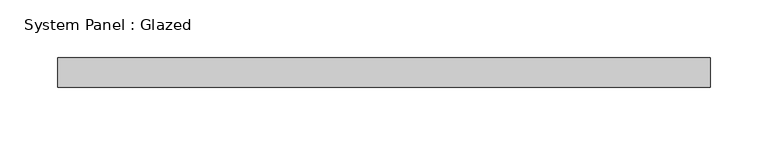
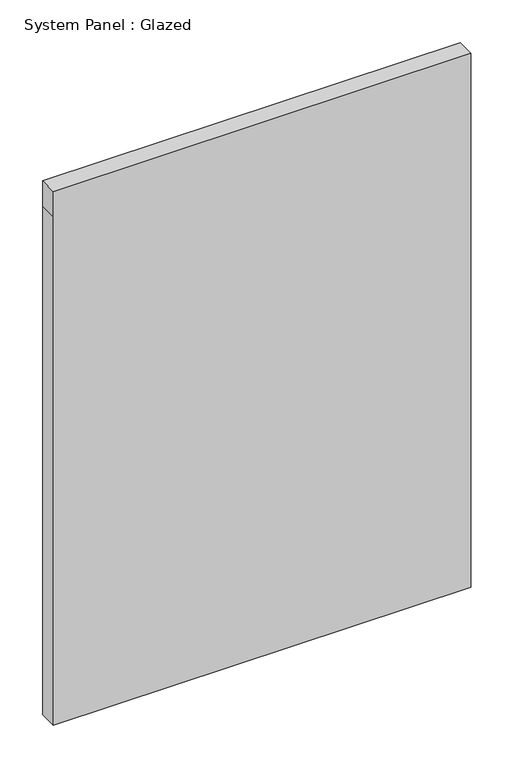
"""IFC4 building model written with IfcOpenShell, lengths in millimetres: plate geometry, System Panel : Glazed."""

from ifc_helpers import new_model, si_unit, frame, origin, place, context, project, spatial, polyline, outline, extrude, source, transform, mapped, element, save


def system_panel_glazed_6bcf57a8(model_context):
    return source(origin(), model_context, "Body", "SweptSolid", [
        extrude(outline(polyline([(0.0, -282.575), (0.0, 282.575), (727.7941631, 282.575), (763.7774964, 282.575), (763.7774964, -282.575), (727.7941631, -282.575), (0.0, -282.575)])), frame((0.0, 19.05, 0.0), z_axis=(0.0, 1.0, 0.0), x_axis=(0.0, 0.0, 1.0)), (0.0, 0.0, 1.0), 25.4),
    ])


if __name__ == "__main__":
    model = new_model("IFC4")
    model_context = context("Model", 3, world=origin())
    ifc_project = project(units=[si_unit("LENGTHUNIT", "METRE", prefix="MILLI")], contexts=[model_context])
    site = spatial("IfcSite", under=ifc_project)
    building = spatial("IfcBuilding", under=site)
    placement = place(None, origin())
    system_panel_glazed_shape = system_panel_glazed_6bcf57a8(model_context)
    element("IfcPlate", 1, ObjectType="System Panel : Glazed", at=placement, inside=building, context=model_context, shape_type="MappedRepresentation", body=[
        mapped(system_panel_glazed_shape, transform((0.0, 0.0, 0.0), x_axis=(1.0, 0.0, 0.0), y_axis=(0.0, 1.0, 0.0), z_axis=(0.0, 0.0, 1.0))),
    ])
    save(model, "model.ifc")

# Revit data of these elements
# Type "System Panel : Glazed"
#   Construction Type Id = "GSP4R"
#   Analytic Construction = "1/8 in Pilkington single glazing"
#   Visual Light Transmittance = 0.9
#   Solar Heat Gain Coefficient = 0.86
#   Heat Transfer Coefficient (U) = 1.18115 BTU/(h·ft²·°F)
#   Define Thermal Properties by = 1
# Element 1 (IfcPlate, "System Panel : Glazed")
#   Materials on its faces: "Glass"
# Materials
#   "Glass": class "Glass", colour RGB 0 128 192, transparency 0.75, Description = "Soda Lime Glass", Cost = 0
